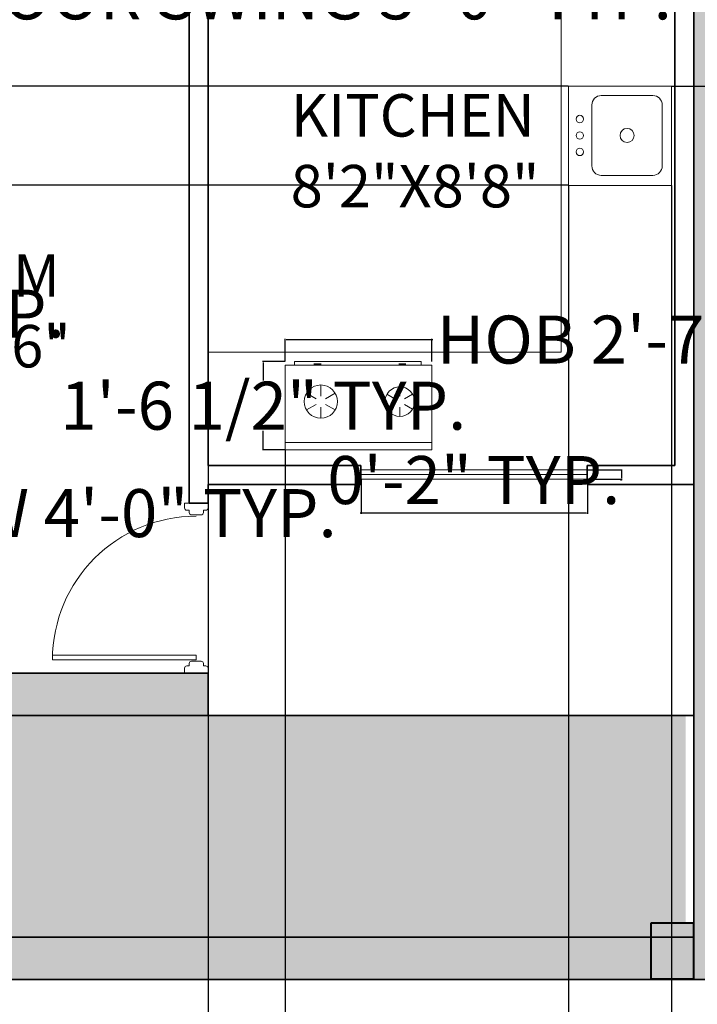
# Model space of a CAD drawing. Units: inches. Extents: x 1077 to 2505, y 1892 to 2728.
# Tile 21 of 26: x 2147 to 2291, y 2089 to 2298. Entities that reach past the tile are written whole.
import ezdxf

# ---------------------------------------------------------------- set-up
doc = ezdxf.new("R2010")
doc.units = ezdxf.units.IN
doc.linetypes.add('ACAD_ISO02W100', pattern=[15, 12, -3])
doc.layers.get('Defpoints').update_dxf_attribs({"color": 220, "linetype": 'ACAD_ISO02W100'})
for name, color, linetype, lineweight in [('00 FURNITURE', 15, 'Continuous', 15), ('A-ANNO-DIMS', 2, 'Continuous', 18), ('A-AREA-IDEN', 7, 'Continuous', 18), ('A-COLS', 7, 'Continuous', 40), ('A-DOOR', 4, 'Continuous', 18), ('A-EQPM', 8, 'Continuous', 13), ('A-FLOR-CASE', 8, 'Continuous', 18), ('A-FLOR-FIXT', 8, 'Continuous', 13), ('A-WALL-PATT', 7, 'Continuous', 9), ('A_TEXT_SMALL', 18, 'Continuous', 13), ('WALL', 7, 'Continuous', 35), ('WINDOW', 160, 'Continuous', 13)]:
    doc.layers.add(name, color=color, linetype=linetype, lineweight=lineweight)
for name, color, linetype, lineweight, true_color in [('A-FLOR-PATT', 254, 'Continuous', 9, 0xd7ebd2), ('FURN3D', 229, 'Continuous', 5, 0x4a3f41), ('L-PLNT-PATT', 116, 'Continuous', 9, 0x136734)]:
    doc.layers.add(name, color=color, linetype=linetype, lineweight=lineweight, true_color=true_color)
doc.styles.get("Standard").update_dxf_attribs({"font": 'arial.ttf'})
doc.dimstyles.get("Standard").update_dxf_attribs({"dimtxt": 10.18, "dimasz": 0.18, "dimexe": 0.18, "dimexo": 0.0625, "dimgap": 0.09, "dimtad": 0, "dimtih": 1, "dimtoh": 1, "dimdec": 0, "dimzin": 0, "dimdsep": 46, "dimlunit": 3, "dimtxsty": 'Standard', "dimcen": 0.09, "dimadec": 0, "dimazin": 0, "dimtfac": 1, "dimtdec": 0, "dimtofl": 0, "dimtmove": 0, "dimatfit": 3, "dimfxl": 1, "dimtolj": 1, "dimtzin": 0, "dimarcsym": 0})

# ---------------------------------------------------------------- blocks, each defined once
blk = doc.blocks.new('DDD')
at = {"layer": '00 FURNITURE'}
for p, q in [((-12579.77, -15859.53), (-12579.77, -15829.05)), ((-12578.77, -15859.53), (-12578.77, -15829.03)), ((-12612.02, -15857.03), (-12612.02, -15862.03)), ((-12611.02, -15857.03), (-12612.02, -15857.03)), ((-12610.52, -15858.03), (-12610.52, -15857.53)), ((-12577.52, -15858.03), (-12577.52, -15857.53)), ((-12577.02, -15857.03), (-12576.02, -15857.03)), ((-12576.02, -15857.03), (-12576.02, -15862.03)), ((-12610.52, -15861.53), (-12610.52, -15861.03)), ((-12578.77, -15859.53), (-12579.77, -15859.53)), ((-12577.52, -15861.53), (-12577.52, -15861.03)), ((-12612.02, -15862.03), (-12611.02, -15862.03)), ((-12576.02, -15862.03), (-12577.02, -15862.03))]:
    blk.add_line(p, q, dxfattribs=at)
for points in [[(-12610.52, -15861.03), (-12610.02, -15861.03, 0.414214), (-12609.52, -15860.53), (-12609.52, -15858.53, 0.414214), (-12610.02, -15858.03), (-12610.52, -15858.03)], [(-12577.52, -15861.03), (-12578.02, -15861.03, -0.414214), (-12578.52, -15860.53), (-12578.52, -15858.53, -0.414214), (-12578.02, -15858.03), (-12577.52, -15858.03)]]:
    blk.add_lwpolyline(points, format="xyb", dxfattribs=at)
for centre, radius, start, end in [((-12578.77, -15859.53), 30.5, 90, 180), ((-12611.02, -15857.53), 0.5, 0, 90), ((-12577.02, -15857.53), 0.5, 90, 180), ((-12611.02, -15861.53), 0.5, 270, 0), ((-12577.02, -15861.53), 0.5, 180, 270)]:
    blk.add_arc(centre, radius, start, end, dxfattribs=at)
blk = doc.blocks.new('A$C21540130')
at = {"layer": 'FURN3D'}
for p, q in [((1.57, 0), (1.57, 31.11)), ((9.61, 25.31), (8.63, 27.01)), ((10.79, 25.31), (11.77, 27.01)), ((9.02, 24.29, -27.54), (7.06, 24.29, -27.54)), ((9.61, 23.27), (8.63, 21.57)), ((10.79, 23.27), (11.77, 21.57)), ((11.38, 24.29, -27.54), (13.34, 24.29, -27.54)), ((9.61, 8.56), (8.43, 10.6)), ((10.79, 8.56), (11.97, 10.6)), ((9.02, 7.54), (6.67, 7.54)), ((9.61, 6.52), (8.43, 4.48)), ((10.79, 6.52), (11.97, 4.48)), ((11.38, 7.54), (13.73, 7.54))]:
    blk.add_line(p, q, dxfattribs=at)
for points in [[(0, 0), (0, 31.11), (17.9, 31.11), (17.9, 0)], [(18.68, 1.96), (18.68, 28.83), (17.9, 28.83), (17.9, 1.96)]]:
    blk.add_lwpolyline(points, close=True, dxfattribs=at)
for centre, radius in [((10.2, 24.29), 3.14), ((10.2, 7.54), 3.53)]:
    blk.add_circle(centre, radius, dxfattribs=at)
for points in [[(17.9, 24.03), (18.29, 24.03), (17.9, 25.6), (18.29, 25.6)], [(17.9, 6.05), (18.29, 6.05), (17.9, 7.62), (18.29, 7.62)]]:
    blk.add_solid(points, dxfattribs=at)
blk = doc.blocks.new('reh-flat-2')
at = {"layer": 'A_TEXT_SMALL'}
for p, q in [((486053827.2, -394630231.2), (486054182.4, -394629799.8)), ((486054182.4, -394629799.8), (486054596.6, -394630140.9)), ((486053979.5, -394630126.3), (486054157.1, -394629910.6)), ((486054228.6, -394629903.6), (486054483.5, -394630113.5)), ((486054596.6, -394630140.9), (486054241.4, -394630572.3)), ((486054241.3, -394630407.7), (486053986.4, -394630197.8)), ((486054490.4, -394630185), (486054312.8, -394630400.7)), ((486054241.4, -394630572.3), (486053827.2, -394630231.2))]:
    blk.add_line(p, q, dxfattribs=at)
for centre, radius in [((486054234.9, -394630155.7), 38.1), ((486054004.1, -394630296.2), 20.1), ((486054072.7, -394630352.7), 20.1), ((486054141.4, -394630409.3), 20.1)]:
    blk.add_circle(centre, radius, dxfattribs=at)
for centre, start, end in [((486054196.3, -394629942.9), 50.5305, 140.5305), ((486054018.7, -394630158.5), 140.5305, 230.5305), ((486054451.2, -394630152.8), 320.5305, 50.5305), ((486054273.6, -394630368.4), 230.5305, 320.5305)]:
    blk.add_arc(centre, 50.8, start, end, dxfattribs=at)
blk = doc.blocks.new('C1')
h = blk.add_hatch(color=256)
h.dxf.hatch_style = 1
h.paths.add_polyline_path([(1668.56, 2445.41), (1677.56, 2445.41), (1677.56, 2457.41), (1668.56, 2457.41)])
for p, q in [((1668.56, 2457.41), (1677.56, 2457.41)), ((1668.56, 2445.41), (1668.56, 2457.41)), ((1677.56, 2457.41), (1677.56, 2445.41)), ((1677.56, 2445.41), (1668.56, 2445.41))]:
    blk.add_line(p, q)
blk = doc.blocks.new('WINDOW-48-PARTITION')
for p, q in [((48, 2), (0, 2)), ((48, 1), (0, 1)), ((48, 0), (0, 0))]:
    blk.add_line(p, q)
blk = doc.blocks.new('*D40')
at = {"layer": 'A-ANNO-DIMS', "color": 0, "lineweight": -2, "transparency": 16777216}
for p, q in [((2203.23, 2225.22), (2203.23, 2230.01)), ((2203.41, 2229.83), (2234.16, 2229.83)), ((2234.34, 2225.22), (2234.34, 2230.01)), ((2234.34, 2229.83), (2234.52, 2229.83))]:
    blk.add_line(p, q, dxfattribs=at)
at = {"layer": 'A-ANNO-DIMS', "color": 0, "transparency": 16777216}
for points in [[(2203.41, 2229.86), (2203.41, 2229.8), (2203.23, 2229.83)], [(2234.16, 2229.86), (2234.16, 2229.8), (2234.34, 2229.83)]]:
    blk.add_solid(points, dxfattribs=at)
at = {"layer": 'Defpoints', "color": 0, "transparency": 16777216}
for p in [(2234.34, 2229.83), (2203.23, 2225.16), (2234.34, 2225.16)]:
    blk.add_point(p, dxfattribs=at)
at = {"layer": 'A-ANNO-DIMS', "color": 0, "transparency": 16777216, "insert": (2282.74, 2229.83), "char_height": 10.18, "attachment_point": 5}
blk.add_mtext('\\A1;HOB 2\'-7" TYP.', dxfattribs=at)
blk = doc.blocks.new('*D41')
at = {"layer": 'A-ANNO-DIMS', "color": 0, "lineweight": -2, "transparency": 16777216}
for p, q in [((2203.17, 2225.16), (2198.39, 2225.16)), ((2198.57, 2224.98), (2198.57, 2221.17)), ((2198.57, 2206.66), (2198.57, 2210.47)), ((2203.17, 2206.48), (2198.39, 2206.48))]:
    blk.add_line(p, q, dxfattribs=at)
at = {"layer": 'A-ANNO-DIMS', "color": 0, "transparency": 16777216}
for points in [[(2198.54, 2224.98), (2198.6, 2224.98), (2198.57, 2225.16)], [(2198.54, 2206.66), (2198.6, 2206.66), (2198.57, 2206.48)]]:
    blk.add_solid(points, dxfattribs=at)
at = {"layer": 'Defpoints', "color": 0, "transparency": 16777216}
for p in [(2198.57, 2225.16), (2203.23, 2225.16), (2203.23, 2206.48)]:
    blk.add_point(p, dxfattribs=at)
at = {"layer": 'A-ANNO-DIMS', "color": 0, "transparency": 16777216, "insert": (2198.57, 2215.82), "char_height": 10.18, "attachment_point": 5}
blk.add_mtext('\\A1;1\'-6 1/2" TYP.', dxfattribs=at)
blk = doc.blocks.new('*D46')
at = {"layer": 'A-ANNO-DIMS', "color": 0, "lineweight": -2, "transparency": 16777216}
for p, q in [((2289.89, 2308.17), (2289.89, 2302.65)), ((2325.89, 2308.17), (2325.89, 2302.65)), ((2289.89, 2302.83), (2289.71, 2302.83)), ((2325.71, 2302.83), (2290.07, 2302.83))]:
    blk.add_line(p, q, dxfattribs=at)
at = {"layer": 'A-ANNO-DIMS', "color": 0, "transparency": 16777216}
for points in [[(2290.07, 2302.86), (2290.07, 2302.8), (2289.89, 2302.83)], [(2325.71, 2302.86), (2325.71, 2302.8), (2325.89, 2302.83)]]:
    blk.add_solid(points, dxfattribs=at)
at = {"layer": 'Defpoints', "color": 0, "transparency": 16777216}
for p in [(2289.89, 2308.23), (2325.89, 2308.23), (2289.89, 2302.83)]:
    blk.add_point(p, dxfattribs=at)
at = {"layer": 'A-ANNO-DIMS', "color": 0, "transparency": 16777216, "insert": (2209.47, 2302.83), "char_height": 10.18, "attachment_point": 5}
blk.add_mtext('\\A1;DOOR SWING 3\'-0" TYP.', dxfattribs=at)
blk = doc.blocks.new('*D50')
at = {"layer": 'A-ANNO-DIMS', "color": 0, "lineweight": -2, "transparency": 16777216}
for p, q in [((2219.31, 2200.18), (2219.31, 2192.86)), ((2267.31, 2200.18), (2267.31, 2192.86)), ((2219.31, 2193.04), (2219.13, 2193.04)), ((2267.13, 2193.04), (2219.49, 2193.04))]:
    blk.add_line(p, q, dxfattribs=at)
at = {"layer": 'A-ANNO-DIMS', "color": 0, "transparency": 16777216}
for points in [[(2219.49, 2193.07), (2219.49, 2193.01), (2219.31, 2193.04)], [(2267.13, 2193.07), (2267.13, 2193.01), (2267.31, 2193.04)]]:
    blk.add_solid(points, dxfattribs=at)
at = {"layer": 'Defpoints', "color": 0, "transparency": 16777216}
for p in [(2219.31, 2200.24), (2267.31, 2200.24), (2219.31, 2193.04)]:
    blk.add_point(p, dxfattribs=at)
at = {"layer": 'A-ANNO-DIMS', "color": 0, "transparency": 16777216, "insert": (2115.19, 2193.04), "char_height": 10.18, "attachment_point": 5}
blk.add_mtext('\\A1;PARTITION WINDOW 4\'-0" TYP.', dxfattribs=at)
blk = doc.blocks.new('*D51')
at = {"layer": 'A-ANNO-DIMS', "color": 0, "lineweight": -2, "transparency": 16777216}
for p, q in [((2267.37, 2202.24), (2274.69, 2202.24)), ((2274.51, 2202.06), (2274.51, 2200.42)), ((2267.37, 2200.24), (2274.69, 2200.24)), ((2274.51, 2200.06), (2274.33, 2200.06)), ((2274.51, 2200.24), (2274.51, 2200.06))]:
    blk.add_line(p, q, dxfattribs=at)
at = {"layer": 'A-ANNO-DIMS', "color": 0, "transparency": 16777216}
for points in [[(2274.48, 2202.06), (2274.54, 2202.06), (2274.51, 2202.24)], [(2274.48, 2200.42), (2274.54, 2200.42), (2274.51, 2200.24)]]:
    blk.add_solid(points, dxfattribs=at)
at = {"layer": 'Defpoints', "color": 0, "transparency": 16777216}
for p in [(2267.31, 2202.24), (2267.31, 2200.24), (2274.51, 2200.24)]:
    blk.add_point(p, dxfattribs=at)
at = {"layer": 'A-ANNO-DIMS', "color": 0, "transparency": 16777216, "insert": (2243.21, 2200.06), "char_height": 10.18, "attachment_point": 5}
blk.add_mtext('\\A1;0\'-2" TYP.', dxfattribs=at)
blk = doc.blocks.new('*D54')
at = {"layer": 'A-ANNO-DIMS', "color": 0, "lineweight": -2, "transparency": 16777216}
for p, q in [((2081.59, 2278.66), (2094.7, 2278.66)), ((2094.52, 2278.48), (2094.52, 2240.71)), ((2094.52, 2192.23), (2094.52, 2230)), ((2081.59, 2192.05), (2094.7, 2192.05))]:
    blk.add_line(p, q, dxfattribs=at)
at = {"layer": 'A-ANNO-DIMS', "color": 0, "transparency": 16777216}
for points in [[(2094.49, 2278.48), (2094.55, 2278.48), (2094.52, 2278.66)], [(2094.49, 2192.23), (2094.55, 2192.23), (2094.52, 2192.05)]]:
    blk.add_solid(points, dxfattribs=at)
at = {"layer": 'Defpoints', "color": 0, "transparency": 16777216}
for p in [(2081.53, 2278.66), (2081.53, 2192.05), (2094.52, 2192.05)]:
    blk.add_point(p, dxfattribs=at)
at = {"layer": 'A-ANNO-DIMS', "color": 0, "transparency": 16777216, "insert": (2094.52, 2235.35), "char_height": 10.18, "attachment_point": 5}
blk.add_mtext('\\A1;SOFA 7\'-2 1/2" TYP.', dxfattribs=at)
blk = doc.blocks.new('*D63')
at = {"layer": 'A-ANNO-DIMS', "color": 0, "lineweight": -2, "transparency": 16777216}
for p, q in [((2035.85, 2094.07), (2035.85, 2065.11)), ((2413.85, 2094.07), (2413.85, 2065.11)), ((2036.03, 2065.29), (2207.27, 2065.29)), ((2413.67, 2065.29), (2242.42, 2065.29))]:
    blk.add_line(p, q, dxfattribs=at)
at = {"layer": 'A-ANNO-DIMS', "color": 0, "transparency": 16777216}
for points in [[(2036.03, 2065.32), (2036.03, 2065.26), (2035.85, 2065.29)], [(2413.67, 2065.32), (2413.67, 2065.26), (2413.85, 2065.29)]]:
    blk.add_solid(points, dxfattribs=at)
at = {"layer": 'Defpoints', "color": 0, "transparency": 16777216}
for p in [(2035.85, 2094.14), (2413.85, 2094.14), (2413.85, 2065.29)]:
    blk.add_point(p, dxfattribs=at)
at = {"layer": 'A-ANNO-DIMS', "color": 0, "transparency": 16777216, "insert": (2224.85, 2065.29), "char_height": 10.18, "attachment_point": 5}
blk.add_mtext('\\A1;31\'-6"', dxfattribs=at)
blk = doc.blocks.new('*D68')
at = {"layer": 'A-ANNO-DIMS', "color": 0, "lineweight": -2, "transparency": 16777216}
for p, q in [((2289.82, 2308.23), (2006.75, 2308.23)), ((2006.93, 2308.05), (2006.93, 2206.47)), ((2006.93, 2094.32), (2006.93, 2195.9)), ((2289.78, 2094.14), (2006.75, 2094.14))]:
    blk.add_line(p, q, dxfattribs=at)
at = {"layer": 'A-ANNO-DIMS', "color": 0, "transparency": 16777216}
for points in [[(2006.9, 2308.05), (2006.96, 2308.05), (2006.93, 2308.23)], [(2006.9, 2094.32), (2006.96, 2094.32), (2006.93, 2094.14)]]:
    blk.add_solid(points, dxfattribs=at)
at = {"layer": 'Defpoints', "color": 0, "transparency": 16777216}
for p in [(2006.93, 2308.23), (2289.89, 2308.23), (2289.85, 2094.14)]:
    blk.add_point(p, dxfattribs=at)
at = {"layer": 'A-ANNO-DIMS', "color": 0, "transparency": 16777216, "insert": (2006.93, 2201.18), "char_height": 10.18, "attachment_point": 5}
blk.add_mtext('\\A1;17\'-10"', dxfattribs=at)
blk = doc.blocks.new('*D69')
at = {"layer": 'A-ANNO-DIMS', "color": 0, "lineweight": -2, "transparency": 16777216}
for p, q in [((2263.27, 2262.49), (2263.27, 2065.11)), ((2285.18, 2262.49), (2285.18, 2065.11)), ((2263.45, 2065.29), (2285, 2065.29)), ((2285.18, 2065.29), (2285.36, 2065.29))]:
    blk.add_line(p, q, dxfattribs=at)
at = {"layer": 'A-ANNO-DIMS', "color": 0, "transparency": 16777216}
for points in [[(2263.45, 2065.32), (2263.45, 2065.26), (2263.27, 2065.29)], [(2285, 2065.32), (2285, 2065.26), (2285.18, 2065.29)]]:
    blk.add_solid(points, dxfattribs=at)
at = {"layer": 'Defpoints', "color": 0, "transparency": 16777216}
for p in [(2263.27, 2262.55), (2285.18, 2262.55), (2285.18, 2065.29)]:
    blk.add_point(p, dxfattribs=at)
at = {"layer": 'A-ANNO-DIMS', "color": 0, "transparency": 16777216, "insert": (2302.45, 2065.29), "char_height": 10.18, "attachment_point": 5}
blk.add_mtext('\\A1;1\'-10"', dxfattribs=at)
blk = doc.blocks.new('*D70')
at = {"layer": 'A-ANNO-DIMS', "color": 0, "lineweight": -2, "transparency": 16777216}
for p, q in [((2263.21, 2283.58), (2006.75, 2283.58)), ((2006.93, 2283.4), (2006.93, 2278.35)), ((2006.93, 2262.73), (2006.93, 2267.78)), ((2263.21, 2262.55), (2006.75, 2262.55))]:
    blk.add_line(p, q, dxfattribs=at)
at = {"layer": 'A-ANNO-DIMS', "color": 0, "transparency": 16777216}
for points in [[(2006.9, 2283.4), (2006.96, 2283.4), (2006.93, 2283.58)], [(2006.9, 2262.73), (2006.96, 2262.73), (2006.93, 2262.55)]]:
    blk.add_solid(points, dxfattribs=at)
at = {"layer": 'Defpoints', "color": 0, "transparency": 16777216}
for p in [(2006.93, 2283.58), (2263.27, 2283.58), (2263.27, 2262.55)]:
    blk.add_point(p, dxfattribs=at)
at = {"layer": 'A-ANNO-DIMS', "color": 0, "transparency": 16777216, "insert": (2006.93, 2273.06), "char_height": 10.18, "attachment_point": 5}
blk.add_mtext('\\A1;1\'-9"', dxfattribs=at)
blk = doc.blocks.new('*D71')
at = {"layer": 'A-ANNO-DIMS', "color": 0, "lineweight": -2, "transparency": 16777216}
for p, q in [((2203.23, 2206.41), (2203.23, 2065.11)), ((2186.85, 2203.07), (2186.85, 2065.11)), ((2187.03, 2065.29), (2203.05, 2065.29)), ((2203.23, 2065.29), (2203.41, 2065.29))]:
    blk.add_line(p, q, dxfattribs=at)
at = {"layer": 'A-ANNO-DIMS', "color": 0, "transparency": 16777216}
for points in [[(2187.03, 2065.32), (2187.03, 2065.26), (2186.85, 2065.29)], [(2203.05, 2065.32), (2203.05, 2065.26), (2203.23, 2065.29)]]:
    blk.add_solid(points, dxfattribs=at)
at = {"layer": 'Defpoints', "color": 0, "transparency": 16777216}
for p in [(2203.23, 2206.48), (2186.85, 2203.14), (2203.23, 2065.29)]:
    blk.add_point(p, dxfattribs=at)
at = {"layer": 'A-ANNO-DIMS', "color": 0, "transparency": 16777216, "insert": (2228.41, 2065.29), "char_height": 10.18, "attachment_point": 5}
blk.add_mtext('\\A1;1\'-4 1/2"', dxfattribs=at)
blk = doc.blocks.new('*D72')
at = {"layer": 'A-ANNO-DIMS', "color": 0, "lineweight": -2, "transparency": 16777216}
for p, q in [((2280.86, 2313.12), (2442.88, 2313.12)), ((2442.7, 2312.94), (2442.7, 2303.7)), ((2442.7, 2283.76), (2442.7, 2292.99)), ((2285.24, 2283.58), (2442.88, 2283.58))]:
    blk.add_line(p, q, dxfattribs=at)
at = {"layer": 'A-ANNO-DIMS', "color": 0, "transparency": 16777216}
for points in [[(2442.67, 2312.94), (2442.73, 2312.94), (2442.7, 2313.12)], [(2442.67, 2283.76), (2442.73, 2283.76), (2442.7, 2283.58)]]:
    blk.add_solid(points, dxfattribs=at)
at = {"layer": 'Defpoints', "color": 0, "transparency": 16777216}
for p in [(2280.8, 2313.12), (2285.18, 2283.58), (2442.7, 2283.58)]:
    blk.add_point(p, dxfattribs=at)
at = {"layer": 'A-ANNO-DIMS', "color": 0, "transparency": 16777216, "insert": (2442.7, 2298.35), "char_height": 10.18, "attachment_point": 5}
blk.add_mtext('\\A1;2\'-5 1/2"', dxfattribs=at)

msp = doc.modelspace()

# ---------------------------------------------------------------- hatches: boundary and pattern name
at = {"layer": 'A-FLOR-PATT', "transparency": 33554559}
h = msp.add_hatch(color=256, dxfattribs=at)
h.dxf.hatch_style = 1
h.paths.add_polyline_path([(2252.85, 2583.14), (2232.15, 2583.14), (2208.15, 2583.17), (2208.15, 2583.14), (2186.85, 2583.14), (2186.85, 2486.14), (2186.85, 2475.14), (2182.85, 2475.14), (2182.85, 2521.11), (2164.84, 2521.11), (2164.84, 2583.14), (2126.63, 2583.14), (2078.63, 2583.13), (2078.63, 2583.14), (2044.85, 2583.14), (2044.85, 2439.14), (2146.85, 2439.14), (2146.85, 2435.14), (2120.85, 2435.14), (2044.85, 2435.14), (2044.85, 2401), (2044.85, 2401), (2044.85, 2377), (2044.85, 2377), (2044.85, 2313.14), (2116.85, 2313.14), (2116.85, 2405.14), (2120.85, 2405.14), (2120.85, 2313.14), (2146.85, 2313.14), (2146.85, 2312.21), (2182.85, 2312.21), (2182.85, 2313.14), (2186.85, 2313.14), (2186.85, 2312.21), (2222.85, 2312.21), (2222.85, 2313.14), (2289.85, 2313.14), (2289.85, 2094.14), (2404.85, 2094.14), (2404.85, 2146.06), (2368.85, 2146.06), (2368.85, 2273.14), (2332.85, 2273.14), (2332.85, 2309.14), (2325.85, 2309.14), (2325.85, 2313.14), (2404.85, 2313.14), (2404.85, 2354.2), (2404.85, 2402.2), (2404.85, 2435.14), (2292.85, 2435.14), (2292.85, 2439.14), (2333.66, 2439.14), (2333.66, 2457.16), (2404.85, 2457.16), (2404.85, 2583.14), (2356.85, 2583.14), (2356.85, 2592.14), (2404.85, 2592.14), (2404.85, 2648.14), (2375.5, 2648.14), (2375.5, 2648.03), (2351.47, 2648.03), (2351.47, 2648.14), (2326.85, 2648.14), (2326.85, 2583.14), (2256.85, 2583.14), (2256.85, 2435.14), (2182.85, 2435.14), (2182.85, 2439.14), (2186.85, 2439.14), (2252.85, 2439.14), (2252.85, 2486.14), (2216.85, 2486.14), (2216.85, 2490.14), (2252.85, 2490.14)])
h.paths.add_polyline_path([(2214.97, 2488.05), (2212.97, 2488.05), (2212.97, 2487.05, 0.414214), (2213.97, 2486.05), (2201.97, 2486.05), (2201.97, 2483.04), (2200.58, 2483.04), (2200.58, 2486.05), (2187.97, 2486.05, -0.414214), (2186.97, 2487.05), (2186.97, 2490.05), (2188.97, 2490.05), (2188.97, 2516.05, -0.446908)], flags=16)
h.paths.add_polyline_path([(2162.4, 2565.16), (2146.2, 2565.16), (2146.2, 2581.36), (2162.4, 2581.36)], flags=16)
h.paths.add_polyline_path([(2161.5, 2566.06), (2147.1, 2566.06), (2147.1, 2580.46), (2161.5, 2580.46)], flags=0)
h.paths.add_polyline_path([(2145.3, 2506.66, -0.414214), (2144.4, 2505.76), (2122.45, 2505.76), (2081.4, 2505.76, -0.414214), (2080.5, 2506.66), (2080.5, 2563.14), (2080.5, 2577.72), (2080.5, 2581.36), (2145.3, 2581.36), (2145.3, 2577.72), (2144.4, 2577.72, -0.414214), (2145.3, 2576.82)], flags=16)
h.paths.add_polyline_path([(2150.3, 2575.03, -1), (2158.24, 2575.03, -1)], flags=0)
h.paths.add_polyline_path([(2150.64, 2575.03, -1), (2157.89, 2575.03, -1)], flags=0)
h.paths.add_polyline_path([(2180.11, 2468.19), (2180.11, 2437.69), (2180.36, 2436.69), (2180.36, 2437.69), (2179.11, 2437.69), (2179.11, 2468.17, 0.404641), (2149.61, 2437.69), (2149.36, 2436.69, -0.414214), (2148.86, 2436.19), (2148.36, 2436.19), (2148.36, 2435.69, -0.414214), (2147.86, 2435.19), (2146.86, 2435.19), (2146.86, 2440.19), (2147.86, 2440.19, -0.414214), (2148.36, 2439.69), (2148.36, 2439.19), (2148.86, 2439.19, -0.414214), (2149.36, 2438.69), (2149.61, 2437.69, -0.414214)], flags=16)
h.paths.add_polyline_path([(2145.14, 2554.26, 0.292232), (2136.49, 2542.78, 0.052719), (2081.25, 2554.26), (2080.6, 2554.26), (2080.6, 2563.14), (2081.25, 2563.14), (2102.73, 2563.14, -0.117785), (2103.09, 2563.91, -0.059418), (2112.19, 2573, -0.379859), (2114.6, 2572.86, -0.02509), (2118.73, 2569.3, -0.025935), (2122.97, 2573, -0.379859), (2125.38, 2572.86, -0.061767), (2134.84, 2563.41, -0.069393), (2135.14, 2563.14), (2145.14, 2563.14)], flags=0)
h.paths.add_polyline_path([(2120.79, 2554.26), (2117.88, 2554.26, -0.015371), (2115.33, 2552.11, -0.429576), (2112.69, 2552.04, -0.016036), (2110.01, 2554.26), (2080.6, 2554.26), (2080.6, 2560.4), (2104.1, 2560.4, 0.055344), (2112.69, 2552.04, 0.331768), (2114.84, 2551.72, 0.027343), (2119.32, 2555.62, 0.00919)], flags=0)
h.paths.add_polyline_path([(2152.88, 2574.32), (2154.19, 2575.07), (2154.19, 2576.58, 0.399698), (2152.71, 2575.03, 0.119004)], flags=0)
h.paths.add_polyline_path([(2152.53, 2575.03, -1), (2156, 2575.03, -1)], flags=0)
h.paths.add_polyline_path([(2154.27, 2574.94), (2154.34, 2574.98), (2154.34, 2575.07), (2154.3, 2575.09), (2154.23, 2574.96)], flags=0)
h.paths.add_polyline_path([(2259.6, 2468.17, -0.414214), (2290.1, 2437.67), (2290.35, 2438.67), (2290.1, 2437.67, 0.404641), (2260.6, 2468.15), (2260.6, 2437.67), (2259.35, 2437.67), (2259.35, 2436.67, -0.414214), (2258.85, 2436.17), (2258.35, 2436.17), (2258.35, 2435.67, -0.414214), (2257.85, 2435.17), (2256.85, 2435.17), (2256.85, 2440.17), (2257.85, 2440.17, -0.414214), (2258.35, 2439.67), (2258.35, 2439.17), (2258.85, 2439.17, -0.414214), (2259.35, 2438.67)], flags=16)
h.paths.add_polyline_path([(2327.48, 2541.19, -0.414214), (2328.38, 2542.09), (2384.85, 2542.09), (2399.43, 2542.09), (2403.08, 2542.09), (2403.08, 2477.29), (2399.43, 2477.29), (2399.43, 2478.19, -0.414214), (2398.53, 2477.29), (2328.38, 2477.29, -0.414214), (2327.48, 2478.19), (2327.48, 2500.14)], flags=16)
h.paths.add_polyline_path([(2340.38, 2542.09, 0.253465), (2337.43, 2532.13, 0.2538), (2327.47, 2529.17)], flags=16)
h.paths.add_polyline_path([(2080.5, 2518.67, 0.253465), (2090.46, 2515.72, 0.2538), (2093.42, 2505.75)], flags=16)
h.paths.add_polyline_path([(2327.09, 2584.7), (2327.09, 2587.7), (2329.09, 2587.7), (2329.09, 2613.7, -0.01951), (2331.09, 2613.66), (2331.09, 2585.7), (2331.09, 2584.7, -0.414214), (2330.09, 2583.7), (2328.09, 2583.7, -0.414214)], flags=16)
h.paths.add_polyline_path([(2239.78, 2404.11), (2252.36, 2404.11), (2252.36, 2405.72), (2239.78, 2405.72)], flags=16)
h.paths.add_polyline_path([(2237.26, 2403.16), (2237.26, 2395.8), (2237.82, 2395.8), (2237.82, 2402.03, -0.41429), (2238.38, 2402.59), (2253.79, 2402.59, -0.414213), (2254.35, 2402.03), (2254.35, 2395.8), (2254.91, 2395.8), (2254.91, 2403.16)], flags=16)
h.paths.add_polyline_path([(2120.69, 2434.12), (2120.69, 2432.12, -0.414214), (2119.69, 2431.12), (2118.69, 2431.12), (2090.73, 2431.12, 0.400854), (2116.69, 2407.02), (2116.69, 2407.12), (2118.69, 2407.12, -0.446908), (2090.69, 2433.12), (2116.69, 2433.12), (2116.69, 2435.12), (2119.69, 2435.12, -0.414214)], flags=16)
h.paths.add_polyline_path([(2262.11, 2404.11), (2274.69, 2404.11), (2274.69, 2405.72), (2262.11, 2405.72)], flags=16)
h.paths.add_polyline_path([(2259.59, 2403.16), (2262.11, 2404.11), (2274.69, 2404.11), (2277.24, 2403.16)], flags=16)
h.paths.add_polyline_path([(2289.58, 2389.14), (2289.58, 2376.57), (2291.19, 2376.57), (2291.19, 2389.14)], flags=16)
h.paths.add_polyline_path([(2288.62, 2391.67), (2281.15, 2391.67), (2281.15, 2391.11), (2287.5, 2391.11, -0.41429), (2288.06, 2390.54), (2288.06, 2375.14, -0.414237), (2287.5, 2374.58), (2281.15, 2374.58), (2281.15, 2374.01), (2288.62, 2374.01)], flags=16)
h.paths.add_polyline_path([(2274.69, 2357.14), (2274.69, 2355.52), (2276.22, 2355.52, 0.414236), (2277.24, 2356.54), (2277.24, 2358.09)], flags=16)
h.paths.add_polyline_path([(2252.36, 2357.14), (2252.36, 2355.52), (2253.89, 2355.52, 0.414235), (2254.91, 2356.54), (2254.91, 2358.09)], flags=16)
h.paths.add_polyline_path([(2224.02, 2376.03), (2222.41, 2376.03), (2222.41, 2374.5, 0.414235), (2223.43, 2373.48), (2224.98, 2373.48)], flags=16)
h.paths.add_polyline_path([(2276.68, 2365.45), (2276.68, 2359.22, -0.41419), (2276.12, 2358.66), (2260.71, 2358.66, -0.414137), (2260.15, 2359.22), (2260.15, 2365.45), (2254.35, 2365.45), (2254.35, 2359.22, -0.414189), (2253.79, 2358.66), (2238.38, 2358.66, -0.414137), (2237.82, 2359.22), (2237.82, 2365.45)], flags=16)
h.paths.add_polyline_path([(2079.6, 2565.16), (2063.4, 2565.16), (2063.4, 2581.36), (2079.6, 2581.36)], flags=16)
h.paths.add_polyline_path([(2078.7, 2566.06), (2064.3, 2566.06), (2064.3, 2580.46), (2078.7, 2580.46)], flags=0)
h.paths.add_polyline_path([(2339.31, 2583.7), (2339.31, 2586.71), (2340.7, 2586.71), (2340.7, 2583.7), (2342.09, 2583.7), (2342.09, 2580.7), (2340.7, 2580.7), (2340.7, 2583.7)], flags=16)
h.paths.add_polyline_path([(2123.69, 2421.51), (2123.69, 2420.12), (2120.69, 2420.12), (2120.69, 2421.51), (2117.68, 2421.51), (2117.68, 2422.89), (2120.69, 2422.89), (2120.69, 2421.51)], flags=16)
h.paths.add_polyline_path([(2067.57, 2575.03, -1), (2075.51, 2575.03, -1)], flags=0)
h.paths.add_polyline_path([(2067.92, 2575.03, -1), (2075.17, 2575.03, -1)], flags=0)
h.paths.add_polyline_path([(2070.16, 2574.32), (2071.47, 2575.07), (2071.47, 2576.58, 0.399698), (2069.99, 2575.03, 0.119004)], flags=0)
h.paths.add_polyline_path([(2069.81, 2575.03, -1), (2073.28, 2575.03, -1)], flags=0)
h.paths.add_polyline_path([(2071.54, 2574.94), (2071.62, 2574.89), (2071.62, 2574.98)], flags=0)
h.paths.add_polyline_path([(2364.5, 2486.1, 0.052719), (2375.98, 2541.34), (2375.98, 2541.99), (2384.85, 2541.99), (2384.85, 2541.34), (2384.85, 2519.86, -0.117785), (2385.62, 2519.51, -0.059418), (2394.72, 2510.41, -0.379859), (2394.58, 2507.99, -0.02509), (2391.01, 2503.87, -0.025935), (2394.72, 2499.62, -0.379859), (2394.58, 2497.21, -0.061767), (2385.12, 2487.75, -0.069393), (2384.85, 2487.45), (2384.85, 2477.45), (2375.98, 2477.45, 0.292232)], flags=0)
h.paths.add_polyline_path([(2373.75, 2509.9, -0.016036), (2375.98, 2512.58), (2375.98, 2541.99), (2382.12, 2541.99), (2382.12, 2518.49, 0.055344), (2373.75, 2509.9, 0.331768), (2373.44, 2507.75, 0.027343), (2377.33, 2503.27, 0.00919), (2375.98, 2501.8), (2375.98, 2504.71, -0.015371), (2373.82, 2507.26, -0.429576)], flags=0)
h.paths.add_polyline_path([(2356.95, 2631.48, -0.171636), (2360.13, 2636.99), (2360.13, 2639.35), (2356, 2639.35, -0.414214), (2355.01, 2640.34), (2355.01, 2646.64, -0.414214), (2356, 2647.62), (2372.14, 2647.62, -0.414214), (2373.13, 2646.64), (2373.13, 2640.34, -0.414214), (2372.14, 2639.35), (2368.01, 2639.35), (2368.01, 2636.99, -0.171636), (2371.2, 2631.48, -0.258205), (2366.63, 2620.45), (2361.51, 2620.45, -0.258205)], flags=16)
h.paths.add_polyline_path([(2358.52, 2631.48, -0.171636), (2361.71, 2636.99), (2366.43, 2636.99, -0.171636), (2369.62, 2631.48, -0.210384), (2366.67, 2622), (2361.47, 2622, -0.210384)], flags=0)
h.paths.add_polyline_path([(2386.88, 2542.99), (2386.88, 2559.19), (2403.08, 2559.19), (2403.08, 2542.99)], flags=16)
h.paths.add_polyline_path([(2387.78, 2543.89), (2387.78, 2558.29), (2402.18, 2558.29), (2402.18, 2543.89)], flags=0)
h.paths.add_polyline_path([(2392.77, 2551.05, -1), (2400.71, 2551.05, -1)], flags=0)
h.paths.add_polyline_path([(2393.11, 2551.05, -1), (2400.37, 2551.05, -1)], flags=0)
h.paths.add_polyline_path([(2386.88, 2476.39), (2403.08, 2476.39), (2403.08, 2460.19), (2386.88, 2460.19)], flags=16)
h.paths.add_polyline_path([(2398.48, 2550.97), (2398.3, 2550.97, -0.544606), (2396.03, 2549.66), (2395.94, 2549.51, 0.547962)], flags=0)
h.paths.add_polyline_path([(2387.78, 2475.49), (2402.18, 2475.49), (2402.18, 2461.09), (2387.78, 2461.09)], flags=0)
h.paths.add_polyline_path([(2396.79, 2551.12), (2396.74, 2551.2), (2396.7, 2551.12)], flags=0)
h.paths.add_polyline_path([(2400.71, 2468.32, -1), (2392.77, 2468.32, -1)], flags=0)
h.paths.add_polyline_path([(2400.37, 2468.32, -1), (2393.11, 2468.32, -1)], flags=0)
h.paths.add_polyline_path([(2398.48, 2468.25), (2398.3, 2468.25, -0.544606), (2396.03, 2466.94), (2395.94, 2466.78, 0.547962)], flags=0)
h.paths.add_polyline_path([(2396.79, 2468.4), (2396.74, 2468.48), (2396.7, 2468.4)], flags=0)
h.paths.add_polyline_path([(2292.64, 2341.23, -0.414214), (2323.14, 2310.73), (2323.39, 2311.73), (2323.14, 2310.73, 0.404641), (2293.64, 2341.21), (2293.64, 2310.73), (2292.39, 2310.73), (2292.39, 2309.73, -0.414214), (2291.89, 2309.23), (2291.39, 2309.23), (2291.39, 2308.73, -0.414214), (2290.89, 2308.23), (2289.89, 2308.23), (2289.89, 2313.23), (2290.89, 2313.23, -0.414214), (2291.39, 2312.73), (2291.39, 2312.23), (2291.89, 2312.23, -0.414214), (2292.39, 2311.73)], flags=16)
h.paths.add_polyline_path([(2389.45, 2641.69), (2392.75, 2641.69), (2392.75, 2641.87), (2389.45, 2641.87)], flags=16)
edge = h.paths.add_edge_path(flags=16)
edge.add_arc((2393.3, 2638.65), 0.183, 270, 360)
edge.add_line((2393.49, 2638.65), (2393.49, 2645.8))
edge.add_line((2393.49, 2645.8), (2395.61, 2645.8))
edge.add_line((2395.61, 2645.8), (2395.61, 2647.8))
edge.add_line((2395.61, 2647.8), (2390.57, 2647.8))
edge.add_line((2390.57, 2647.8), (2390.57, 2645.8))
edge.add_line((2390.57, 2645.8), (2392.19, 2645.8))
edge.add_line((2392.19, 2645.8), (2392.19, 2644.98))
edge.add_line((2392.19, 2644.98), (2391.02, 2644.98))
edge.add_line((2391.02, 2644.98), (2391.02, 2645.8))
edge.add_line((2391.02, 2645.8), (2390.57, 2645.8))
edge.add_line((2390.57, 2645.8), (2390.57, 2647.8))
edge.add_line((2390.57, 2647.8), (2395.61, 2647.8))
edge.add_line((2395.61, 2647.8), (2395.61, 2647.32))
edge.add_line((2395.61, 2647.32), (2397.95, 2647.56))
edge.add_line((2397.95, 2647.56), (2397.95, 2647.8))
edge.add_line((2397.95, 2647.8), (2398.81, 2647.8))
edge.add_line((2398.81, 2647.8), (2398.81, 2647.23))
edge.add_line((2398.81, 2647.23), (2398.63, 2645.77))
edge.add_ellipse((2398.41, 2644.93), major_axis=(-1.08, 0), ratio=0.790849, start_angle=180, end_angle=255.2976, ccw=False)
edge.add_line((2399.49, 2644.93), (2399.49, 2644.36))
edge.add_ellipse((2398.41, 2644.36), major_axis=(-1.08, 0), ratio=0.790849, start_angle=0, end_angle=180, ccw=False)
edge.add_line((2397.32, 2644.36), (2397.33, 2644.85))
edge.add_ellipse((2398.41, 2644.93), major_axis=(-1.08, 0), ratio=0.790849, start_angle=284.7024, end_angle=364.0401, ccw=False)
edge.add_line((2398.1, 2645.73), (2398.1, 2647.23))
edge.add_line((2398.1, 2647.23), (2397.95, 2647.23))
edge.add_line((2397.95, 2647.23), (2395.61, 2646.99))
edge.add_line((2395.61, 2646.99), (2395.61, 2645.8))
edge.add_line((2395.61, 2645.8), (2393.49, 2645.8))
edge.add_line((2393.49, 2645.8), (2393.49, 2638.46))
edge.add_line((2393.49, 2638.46), (2393.3, 2638.46))
h.paths.add_polyline_path([(2353.64, 2256.32, -0.292371), (2356.22, 2253.81, -0.085148), (2358.52, 2214.83, -0.01331), (2357.59, 2104.48, -0.379287), (2354.54, 2101.26, -0.0502), (2298.86, 2101.26, -0.379287), (2295.81, 2104.48, -0.01331), (2294.88, 2214.83, -0.086132), (2297.28, 2254.24, -0.295116), (2299.9, 2256.76, -0.114238)], flags=16)
h.paths.add_polyline_path([(2352.48, 2211.82, -0.355389), (2354.02, 2208.08), (2350.26, 2195.63, -0.398275), (2346.44, 2193.45, 0.113332), (2306.96, 2193.45, -0.398275), (2303.14, 2195.63), (2299.38, 2208.08, -0.355394), (2300.92, 2211.82, -0.265725)], flags=0)
h.paths.add_polyline_path([(2297.68, 2201.7), (2303.26, 2187.65), (2303.26, 2166.61), (2298.16, 2163.24)], flags=0)
h.paths.add_polyline_path([(2355.78, 2201.7), (2355.31, 2163.24), (2350.2, 2166.61), (2350.2, 2187.65)], flags=0)
h.paths.add_polyline_path([(2303.26, 2164.35), (2303.26, 2143.1), (2298.44, 2128.54), (2298.19, 2161.01)], flags=0)
h.paths.add_polyline_path([(2350.2, 2164.35), (2355.28, 2161.01), (2355.03, 2128.54), (2350.2, 2143.1)], flags=0)
h.paths.add_polyline_path([(2347.2, 2136.38), (2351.71, 2113.65, -0.090102), (2301.76, 2113.63), (2306.27, 2136.37, 0.036636)], flags=0)
h.paths.add_polyline_path([(2304.86, 2165.32), (2354.76, 2165.32), (2354.76, 2183.87), (2304.86, 2183.87)], flags=8)
h.paths.add_polyline_path([(2053.76, 2360.82), (2103.97, 2360.82), (2103.97, 2394.41), (2053.76, 2394.41)], flags=24)
h.paths.add_polyline_path([(2153.41, 2366.23), (2211.12, 2366.23), (2211.12, 2399.82), (2153.41, 2399.82)], flags=24)
h.paths.add_polyline_path([(2258.04, 2477.83), (2327.95, 2477.83), (2327.95, 2511.42), (2258.04, 2511.42)], flags=24)
h.paths.add_polyline_path([(2182.1, 2454.46), (2252.27, 2454.46), (2252.27, 2473), (2182.1, 2473)], flags=24)
h.paths.add_polyline_path([(2192.4, 2537.41), (2246.99, 2537.41), (2246.99, 2571), (2192.4, 2571)], flags=24)
h.paths.add_polyline_path([(2083.07, 2465.98), (2152.99, 2465.98), (2152.99, 2499.56), (2083.07, 2499.56)], flags=24)
at = {"layer": 'A-WALL-PATT', "transparency": 33554585}
h = msp.add_hatch(color=256, dxfattribs=at)
h.dxf.hatch_style = 1
h.paths.add_polyline_path([(2044.85, 2429.98), (2035.85, 2429.98), (2035.85, 2401), (2044.85, 2401)])
h.paths.add_polyline_path([(2044.85, 2377), (2035.85, 2377), (2035.85, 2317.47), (2044.85, 2317.47)])
h.paths.add_polyline_path([(2085.45, 2159.14), (2044.85, 2159.14), (2044.85, 2225.64), (2035.85, 2225.64), (2035.85, 2106.16), (2044.85, 2106.16), (2044.85, 2150.14), (2085.45, 2150.14)])
h.paths.add_polyline_path([(2289.85, 2103.14), (2044.85, 2103.14), (2044.85, 2106.16), (2035.85, 2106.16), (2035.85, 2094.14), (2289.85, 2094.14)])
h.paths.add_polyline_path([(2413.85, 2354.2), (2404.85, 2354.2), (2404.85, 2354.2), (2404.85, 2313.14), (2325.85, 2313.14), (2325.85, 2309.14), (2404.85, 2309.14), (2404.85, 2094.14), (2413.85, 2094.14)])
h.paths.add_polyline_path([(2413.85, 2431.09), (2404.85, 2431.09), (2404.85, 2402.2), (2413.85, 2402.2)])
h.paths.add_polyline_path([(2404.85, 2439.14), (2292.85, 2439.14), (2292.85, 2435.14), (2404.85, 2435.14)])
h.paths.add_polyline_path([(2413.85, 2580.36), (2404.85, 2580.36), (2404.85, 2457.16), (2404.87, 2457.16), (2404.87, 2443.09), (2413.85, 2443.09)])
h.paths.add_polyline_path([(2413.85, 2645.09), (2404.85, 2645.09), (2404.85, 2592.36), (2413.85, 2592.36)])
h.paths.add_polyline_path([(2413.85, 2645.09), (2404.85, 2645.09), (2404.85, 2648.14), (2375.5, 2648.14), (2375.5, 2648.03), (2351.5, 2648.03), (2351.5, 2657.03), (2375.47, 2657.03), (2375.47, 2657.14), (2413.85, 2657.14)])
h.paths.add_polyline_path([(2351.47, 2657.14), (2326.92, 2657.14), (2326.92, 2648.14), (2351.47, 2648.14)])
h.paths.add_polyline_path([(2078.63, 2583.14), (2044.92, 2583.14), (2044.92, 2580.01), (2035.92, 2580.01), (2035.92, 2592.14), (2078.63, 2592.14)])
h.paths.add_polyline_path([(2180.39, 2592.14), (2126.63, 2592.14), (2126.63, 2583.14), (2180.39, 2583.14)])
h.paths.add_polyline_path([(2232.16, 2592.17), (2232.16, 2583.17), (2208.16, 2583.17), (2208.15, 2583.17), (2208.15, 2583.14), (2189.39, 2583.14), (2189.39, 2579.98), (2180.39, 2579.98), (2180.39, 2592.14), (2208.15, 2592.14), (2208.16, 2592.14), (2208.16, 2592.17)])
h.paths.add_polyline_path([(2250.27, 2592.14), (2232.16, 2592.14), (2232.16, 2583.14), (2250.27, 2583.14)], flags=17)
h.paths.add_polyline_path([(2326.85, 2648.14), (2326.92, 2657.14), (2317.85, 2657.14), (2317.85, 2592.14), (2250.27, 2592.14), (2250.27, 2583.14), (2252.85, 2583.14), (2252.85, 2490.14), (2216.85, 2490.14), (2216.85, 2486.14), (2252.85, 2486.14), (2252.85, 2439.14), (2186.85, 2439.14), (2182.85, 2439.14), (2182.85, 2435.14), (2256.85, 2435.14), (2256.85, 2583.14), (2326.85, 2583.14)])
h.paths.add_polyline_path([(2044.85, 2580.01), (2035.85, 2580.01), (2035.85, 2441.98), (2044.85, 2441.98)])
at = {"layer": 'A-WALL-PATT', "transparency": 33554559}
h = msp.add_hatch(color=256, dxfattribs=at)
h.dxf.hatch_style = 1
h.paths.add_polyline_path([(2146.85, 2439.14), (2044.78, 2439.14), (2044.78, 2435.14), (2120.85, 2435.14), (2146.85, 2435.14)])
h.paths.add_polyline_path([(2186.85, 2579.98), (2182.85, 2579.98), (2182.85, 2475.14), (2186.85, 2475.14), (2186.85, 2486.14)])
h.paths.add_polyline_path([(2404.83, 2592.14), (2356.85, 2592.14), (2356.85, 2587.7), (2357.09, 2587.7), (2357.09, 2584.7, -0.178139), (2356.85, 2584.05), (2356.85, 2583.14), (2404.83, 2583.14)])
h.paths.add_polyline_path([(2186.85, 2159.14), (2133.45, 2159.14), (2133.45, 2150.14), (2186.85, 2150.14)])
at = {"layer": 'L-PLNT-PATT', "transparency": 33554610}
h = msp.add_hatch(color=256, dxfattribs=at)
h.dxf.hatch_style = 1
h.paths.add_polyline_path([(2288.17, 2150.14), (2135.73, 2150.14), (2135.73, 2149.48), (2084.04, 2149.48), (2084.04, 2150.14), (2044.85, 2150.14), (2044.85, 2106.16), (2044.86, 2106.16), (2044.86, 2103.14), (2280.82, 2103.14), (2280.82, 2106.19), (2288.17, 2106.19)])
h.paths.add_polyline_path([(2067.09, 2127.13), (2154.7, 2127.13), (2154.7, 2145.68), (2067.09, 2145.68)], flags=24)

# ---------------------------------------------------------------- linework, layer by layer
at = {"layer": 'A-FLOR-CASE'}
for p, q in [((2261.78, 2308.99), (2261.78, 2227.18)), ((2261.78, 2227.18), (2186.85, 2227.18)), ((2285.89, 2227.18), (2285.85, 2227.18)), ((2285.89, 2203.18), (2285.89, 2227.18))]:
    msp.add_line(p, q, dxfattribs=at)
at = {"layer": 'WALL'}
for p, q in [((2182.85, 2195.14), (2182.85, 2313.14)), ((2186.85, 2203.14), (2186.85, 2313.14)), ((2289.85, 2094.14), (2289.85, 2313.14)), ((2285.85, 2203.14), (2285.85, 2309.14)), ((2186.85, 2203.14), (2219.27, 2203.14)), ((2219.27, 2199.14), (2219.27, 2203.14)), ((2267.27, 2203.14), (2285.85, 2203.14)), ((2267.27, 2199.14), (2267.27, 2203.14)), ((2186.85, 2199.14), (2219.27, 2199.14)), ((2186.85, 2195.14), (2186.85, 2199.14)), ((2267.27, 2199.14), (2289.85, 2199.14)), ((2182.85, 2195.14), (2186.85, 2195.14)), ((2133.45, 2159.14), (2186.85, 2159.14)), ((2186.85, 2150.14), (2186.85, 2159.14)), ((2133.45, 2150.14), (2289.85, 2150.14)), ((2289.85, 2103.14), (2044.85, 2103.14)), ((2413.85, 2094.14), (2035.85, 2094.14))]:
    msp.add_line(p, q, dxfattribs=at)

# ---------------------------------------------------------------- block references
at = {"layer": 'A-COLS'}
msp.add_blockref('C1', (612.26, -351.22), dxfattribs=at)
at = {"layer": 'A-DOOR', "xscale": -1, "rotation": 90}
msp.add_blockref('DDD', (-13675.17, -10416.87), dxfattribs=at)
at = {"layer": 'A-EQPM', "xscale": -1, "rotation": 270}
msp.add_blockref('A$C21540130', (2203.23, 2206.48), dxfattribs=at)
at = {"layer": 'A-FLOR-FIXT', "xscale": 0.0391972730482577, "yscale": 0.0391972730482577, "zscale": 0.0391972730482577, "rotation": 309.4694759622496}
msp.add_blockref('reh-flat-2', (-167395.5, 24542487.85), dxfattribs=at)
at = {"layer": 'WINDOW', "rotation": 180}
msp.add_blockref('WINDOW-48-PARTITION', (2267.31, 2202.24), dxfattribs=at)

# ---------------------------------------------------------------- texts
at = {"layer": 'A-AREA-IDEN', "char_height": 9, "attachment_point": 1}
for s, insert in [('KITCHEN\\P8\'2"X8\'8"', (2204.38, 2281.88)), ('\\pxi-3,l4,t4;DRG.ROOM\\P10\'6"X12\'6"', (2082.35, 2247.94))]:
    msp.add_mtext_dynamic_manual_height_columns(s, width=128.1076, gutter_width=12.5, heights=[0], dxfattribs=dict(at, insert=insert))

# ---------------------------------------------------------------- dimensions: what is measured, and where the dimension line sits
at = {"layer": 'A-ANNO-DIMS'}
for base, p1, p2, angle, text, picture, middle in [((2289.89, 2302.83), (2325.89, 2308.23), (2289.89, 2308.23), 180, 'DOOR SWING <> TYP.', '*D46', (2209.47, 2302.83)), ((2094.52, 2192.05), (2081.53, 2278.66), (2081.53, 2192.05), 270, 'SOFA <> TYP.', '*D54', (2094.52, 2235.35)), ((2198.57, 2225.16), (2203.23, 2206.48), (2203.23, 2225.16), 90, '<> TYP.', '*D41', (2198.57, 2215.82)), ((2219.31, 2193.04), (2267.31, 2200.24), (2219.31, 2200.24), 180, 'PARTITION WINDOW <> TYP.', '*D50', (2115.19, 2193.04)), ((2274.51, 2200.24), (2267.31, 2202.24), (2267.31, 2200.24), 270, '<> TYP.', '*D51', (2243.21, 2200.06))]:
    dim = msp.add_linear_dim(base=base, p1=p1, p2=p2, angle=angle, text=text, dimstyle='Standard', override={"dimdec": 1, "dimlfac": 1, "dimrnd": 0, "dimzin": 1, "dimdsep": 46, "dimlunit": 4, "dimfrac": 2}, dxfattribs=at)
    dim.commit()
    dim.dimension.update_dxf_attribs({"geometry": picture, "text_midpoint": middle})
for base, p1, p2, picture, middle in [((2442.7, 2283.58), (2280.8, 2313.12), (2285.18, 2283.58), '*D72', (2442.7, 2298.35)), ((2006.93, 2308.23), (2289.85, 2094.14), (2289.89, 2308.23), '*D68', (2006.93, 2201.18)), ((2006.93, 2283.58), (2263.27, 2262.55), (2263.27, 2283.58), '*D70', (2006.93, 2273.06))]:
    dim = msp.add_linear_dim(base=base, p1=p1, p2=p2, angle=90, dimstyle='Standard', override={"dimdec": 1, "dimlfac": 1, "dimrnd": 0, "dimzin": 1, "dimdsep": 46, "dimlunit": 4, "dimfrac": 2}, dxfattribs=at)
    dim.commit()
    dim.dimension.update_dxf_attribs({"geometry": picture, "text_midpoint": middle})
for base, p1, p2, picture, middle in [((2285.18, 2065.29), (2263.27, 2262.55), (2285.18, 2262.55), '*D69', (2302.45, 2065.29)), ((2203.23, 2065.29), (2186.85, 2203.14), (2203.23, 2206.48), '*D71', (2228.41, 2065.29)), ((2413.85, 2065.29), (2035.85, 2094.14), (2413.85, 2094.14), '*D63', (2224.85, 2065.29))]:
    dim = msp.add_linear_dim(base=base, p1=p1, p2=p2, dimstyle='Standard', override={"dimdec": 1, "dimlfac": 1, "dimrnd": 0, "dimzin": 1, "dimdsep": 46, "dimlunit": 4, "dimfrac": 2}, dxfattribs=at)
    dim.commit()
    dim.dimension.update_dxf_attribs({"geometry": picture, "text_midpoint": middle})
dim = msp.add_linear_dim(base=(2234.34, 2229.83), p1=(2203.23, 2225.16), p2=(2234.34, 2225.16), text='HOB <> TYP.', dimstyle='Standard', override={"dimdec": 1, "dimlfac": 1, "dimrnd": 0, "dimzin": 1, "dimdsep": 46, "dimlunit": 4, "dimfrac": 2}, dxfattribs=at)
dim.commit()
dim.dimension.update_dxf_attribs({"geometry": '*D40', "text_midpoint": (2282.74, 2229.83)})

doc.saveas('drawing.dxf')
